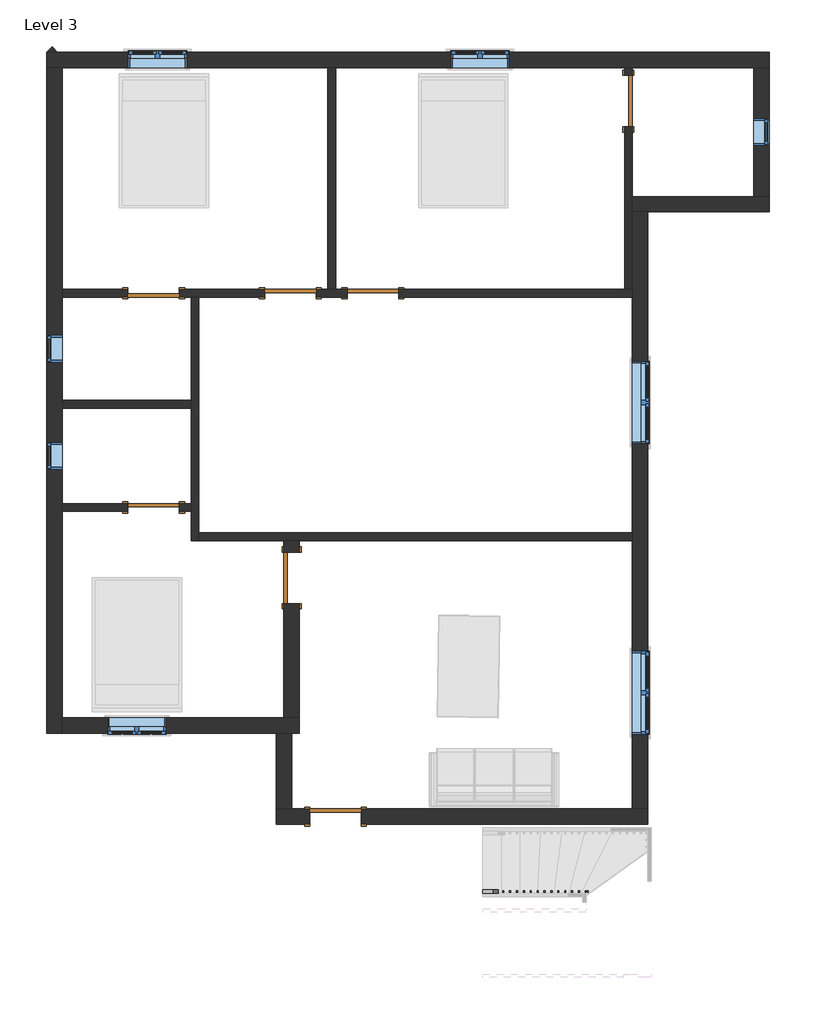
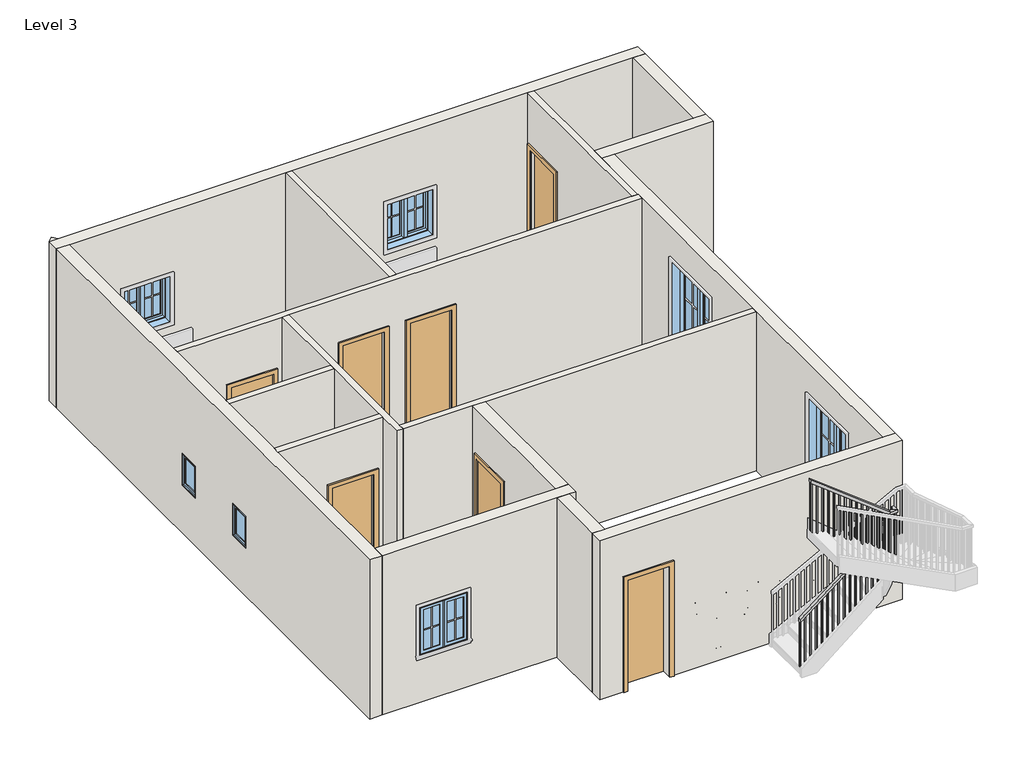
# One storey, part 1 of 2: 17 walls, 8 windows, 7 doors, 1 railing.
"""IFC4 building model written with IfcOpenShell, lengths in millimetres."""

from ifc_helpers import new_model, si_unit, frame, origin, place, context, project, spatial, polyline, outline, extrude, faceted_brep, transform, mapped, element, save
from components import door_f2b275c1, door_d8f5dbb5, door_214872d5, door_78caadf7, door_bb98abfd, window_aa618e30, window_339605e1, window_8377141f

model = new_model("IFC4")

# Units and contexts
model_context = context("Model", 3, world=origin())
ifc_project = project(units=[si_unit("LENGTHUNIT", "METRE", prefix="MILLI")], contexts=[model_context])

# Site, building, storey
site = spatial("IfcSite", under=ifc_project)
building = spatial("IfcBuilding", under=site)
storey = spatial("IfcBuildingStorey", under=building, Name="Level 3", Elevation=3200.4)

# Doors
placement = place(None, origin())
door_shape = door_f2b275c1(model_context)
element("IfcDoor", 1, ObjectType="Single-Flush : 30\" x 80\"", at=placement, inside=storey, context=model_context, shape_type="MappedRepresentation", body=[
    mapped(door_shape, transform((2459.5084916, 7319.9935985, 3200.4), x_axis=(0.0, 1.0, 0.0), y_axis=(-1.0, 0.0, 0.0), z_axis=(0.0, 0.0, 1.0))),
])
element("IfcDoor", 2, ObjectType="Single-Flush : 30\" x 80\"", at=placement, inside=storey, context=model_context, shape_type="MappedRepresentation", body=[
    mapped(door_shape, transform((-4550.8915084, 4481.5435985, 3200.4), x_axis=(1.0, 0.0, 0.0), y_axis=(0.0, 1.0, 0.0), z_axis=(0.0, 0.0, 1.0))),
])
door_2_shape = door_d8f5dbb5(model_context)
element("IfcDoor", 3, ObjectType="Single-Flush : 30\" x 80\"", at=placement, inside=storey, context=model_context, shape_type="MappedRepresentation", body=[
    mapped(door_2_shape, transform((-4550.8915084, 1319.2435985, 3200.4), x_axis=(1.0, 0.0, 0.0), y_axis=(0.0, 1.0, 0.0), z_axis=(0.0, 0.0, 1.0))),
])
door_3_shape = door_214872d5(model_context)
element("IfcDoor", 4, ObjectType="Single-Flush : 30\" x 84\"", at=placement, inside=storey, context=model_context, shape_type="MappedRepresentation", body=[
    mapped(door_3_shape, transform((-2531.5915084, 4481.5435985, 3200.4), x_axis=(1.0, 0.0, 0.0), y_axis=(0.0, 1.0, 0.0), z_axis=(0.0, 0.0, 1.0))),
])
door_4_shape = door_78caadf7(model_context)
element("IfcDoor", 5, ObjectType="Single-Flush : 30\" x 84\"", at=placement, inside=storey, context=model_context, shape_type="MappedRepresentation", body=[
    mapped(door_4_shape, transform((-1312.3915084, 4481.5435985, 3200.4), x_axis=(-1.0, 0.0, 0.0), y_axis=(0.0, -1.0, 0.0), z_axis=(0.0, 0.0, 1.0))),
])
door_5_shape = door_bb98abfd(model_context)
element("IfcDoor", 6, ObjectType="Single-Flush : 30\" x 84\"", at=placement, inside=storey, context=model_context, shape_type="MappedRepresentation", body=[
    mapped(door_5_shape, transform((-2512.5415084, 277.8435985, 3200.4), x_axis=(0.0, 1.0, 0.0), y_axis=(-1.0, 0.0, 0.0), z_axis=(0.0, 0.0, 1.0))),
])
element("IfcDoor", 7, ObjectType="Single-Flush : 30\" x 84\"", at=placement, inside=storey, context=model_context, shape_type="MappedRepresentation", body=[
    mapped(door_5_shape, transform((-1864.8415084, -3246.4064015, 3200.4), x_axis=(1.0, 0.0, 0.0), y_axis=(0.0, 1.0, 0.0), z_axis=(0.0, 0.0, 1.0))),
])

# Railing
element("IfcRailing", 8, ObjectType="Handrail - Rectangular", at=placement, inside=storey, context=model_context, shape_type="SolidModel", body=[
    faceted_brep([(306.9570026, -4325.9064015, 4284.1333333), (306.9570026, -4325.9064015, 4219.8000346), (306.9570026, -4376.7064015, 4219.8000346), (306.9570026, -4376.7064015, 4284.1333333), (1758.4886944, -4325.9064015, 5412.0191036), (1809.2886944, -4325.9064015, 5387.1590024), (1809.2886944, -4376.7064015, 5387.1590024), (1758.4886944, -4376.7064015, 5412.0191036), (1758.4886944, -4325.9064015, 5615.0281882), (1809.2886944, -4325.9064015, 5564.2281882), (1809.2886944, -4376.7064015, 5564.2281882), (1758.4886944, -4376.7064015, 5615.0281882), (1885.4886944, -4325.9064015, 5615.0281882), (1885.4886944, -4325.9064015, 5564.2281882), (1834.6886944, -4376.7064015, 5564.2281882), (1834.6886944, -4376.7064015, 5615.0281882), (1885.4886944, -4452.9064015, 5615.0281882), (1885.4886944, -4482.0277354, 5564.2281882), (1834.6886944, -4482.0277354, 5564.2281882), (1834.6886944, -4452.9064015, 5615.0281882), (1885.4886944, -4579.9064015, 5831.9051451), (1885.4886944, -4630.7064015, 5818.1256424), (1834.6886944, -4630.7064015, 5818.1256424), (1834.6886944, -4579.9064015, 5831.9051451), (1885.4886944, -4579.9064015, 6034.9142297), (1885.4886944, -4630.7064015, 5984.1142297), (1834.6886944, -4630.7064015, 5984.1142297), (1834.6886944, -4579.9064015, 6034.9142297), (1885.4886944, -4706.9064015, 6034.9142297), (1885.4886944, -4706.9064015, 5984.1142297), (1834.6886944, -4656.1064015, 5984.1142297), (1834.6886944, -4656.1064015, 6034.9142297), (1758.4886944, -4706.9064015, 6034.9142297), (1741.0720265, -4706.9064015, 5984.1142297), (1741.0720265, -4656.1064015, 5984.1142297), (1758.4886944, -4656.1064015, 6034.9142297), (306.9570026, -4706.9064015, 7162.8), (306.9570026, -4656.1064015, 7162.8), (306.9570026, -4656.1064015, 7098.4667013), (306.9570026, -4706.9064015, 7098.4667013)], [[[0, 1, 2, 3]], [[1, 0, 4, 5]], [[2, 1, 5, 6]], [[3, 2, 6, 7]], [[0, 3, 7, 4]], [[5, 4, 8, 9]], [[6, 5, 9, 10]], [[7, 6, 10, 11]], [[4, 7, 11, 8]], [[9, 8, 12, 13]], [[10, 9, 13, 14]], [[11, 10, 14, 15]], [[8, 11, 15, 12]], [[13, 12, 16, 17]], [[14, 13, 17, 18]], [[15, 14, 18, 19]], [[12, 15, 19, 16]], [[17, 16, 20, 21]], [[18, 17, 21, 22]], [[19, 18, 22, 23]], [[16, 19, 23, 20]], [[21, 20, 24, 25]], [[22, 21, 25, 26]], [[23, 22, 26, 27]], [[20, 23, 27, 24]], [[25, 24, 28, 29]], [[26, 25, 29, 30]], [[27, 26, 30, 31]], [[24, 27, 31, 28]], [[29, 28, 32, 33]], [[30, 29, 33, 34]], [[31, 30, 34, 35]], [[28, 31, 35, 32]], [[36, 37, 38, 39]], [[33, 32, 36, 39]], [[34, 33, 39, 38]], [[35, 34, 38, 37]], [[32, 35, 37, 36]]]),
    extrude(outline(polyline([(7068.4292361, 345.6136944), (7083.2316852, 326.5636944), (6079.0666667, 326.5636944), (6079.0666667, 345.6136944), (7068.4292361, 345.6136944)])), frame((0.0, -4691.0314015, 0.0), z_axis=(0.0, 1.0, 0.0), x_axis=(0.0, 0.0, 1.0)), (0.0, 0.0, 1.0), 19.05),
    extrude(outline(polyline([(6989.4828411, 447.2136944), (7004.2852902, 428.1636944), (6079.0666667, 428.1636944), (6079.0666667, 447.2136944), (6989.4828411, 447.2136944)])), frame((0.0, -4691.0314015, 0.0), z_axis=(0.0, 1.0, 0.0), x_axis=(0.0, 0.0, 1.0)), (0.0, 0.0, 1.0), 19.05),
    extrude(outline(polyline([(6910.5364462, 548.8136944), (6925.3388952, 529.7636944), (6079.0666667, 529.7636944), (6079.0666667, 548.8136944), (6910.5364462, 548.8136944)])), frame((0.0, -4691.0314015, 0.0), z_axis=(0.0, 1.0, 0.0), x_axis=(0.0, 0.0, 1.0)), (0.0, 0.0, 1.0), 19.05),
    extrude(outline(polyline([(6831.5900512, 650.4136944), (6846.3925003, 631.3636944), (5909.7333333, 631.3636944), (5909.7333333, 650.4136944), (6831.5900512, 650.4136944)])), frame((0.0, -4691.0314015, 0.0), z_axis=(0.0, 1.0, 0.0), x_axis=(0.0, 0.0, 1.0)), (0.0, 0.0, 1.0), 19.05),
    extrude(outline(polyline([(6752.6436562, 752.0136944), (6767.4461053, 732.9636944), (5909.7333333, 732.9636944), (5909.7333333, 752.0136944), (6752.6436562, 752.0136944)])), frame((0.0, -4691.0314015, 0.0), z_axis=(0.0, 1.0, 0.0), x_axis=(0.0, 0.0, 1.0)), (0.0, 0.0, 1.0), 19.05),
    extrude(outline(polyline([(6673.6972613, 853.6136944), (6688.4997103, 834.5636944), (5909.7333333, 834.5636944), (5909.7333333, 853.6136944), (6673.6972613, 853.6136944)])), frame((0.0, -4691.0314015, 0.0), z_axis=(0.0, 1.0, 0.0), x_axis=(0.0, 0.0, 1.0)), (0.0, 0.0, 1.0), 19.05),
    extrude(outline(polyline([(6594.7508663, 955.2136944), (6609.5533154, 936.1636944), (5740.4, 936.1636944), (5740.4, 955.2136944), (6594.7508663, 955.2136944)])), frame((0.0, -4691.0314015, 0.0), z_axis=(0.0, 1.0, 0.0), x_axis=(0.0, 0.0, 1.0)), (0.0, 0.0, 1.0), 19.05),
    extrude(outline(polyline([(6515.8044713, 1056.8136944), (6530.6069204, 1037.7636944), (5740.4, 1037.7636944), (5740.4, 1056.8136944), (6515.8044713, 1056.8136944)])), frame((0.0, -4691.0314015, 0.0), z_axis=(0.0, 1.0, 0.0), x_axis=(0.0, 0.0, 1.0)), (0.0, 0.0, 1.0), 19.05),
    extrude(outline(polyline([(6436.8580764, 1158.4136944), (6451.6605254, 1139.3636944), (5571.0666667, 1139.3636944), (5571.0666667, 1158.4136944), (6436.8580764, 1158.4136944)])), frame((0.0, -4691.0314015, 0.0), z_axis=(0.0, 1.0, 0.0), x_axis=(0.0, 0.0, 1.0)), (0.0, 0.0, 1.0), 19.05),
    extrude(outline(polyline([(6357.9116814, 1260.0136944), (6372.7141304, 1240.9636944), (5571.0666667, 1240.9636944), (5571.0666667, 1260.0136944), (6357.9116814, 1260.0136944)])), frame((0.0, -4691.0314015, 0.0), z_axis=(0.0, 1.0, 0.0), x_axis=(0.0, 0.0, 1.0)), (0.0, 0.0, 1.0), 19.05),
    extrude(outline(polyline([(6278.9652864, 1361.6136944), (6293.7677355, 1342.5636944), (5571.0666667, 1342.5636944), (5571.0666667, 1361.6136944), (6278.9652864, 1361.6136944)])), frame((0.0, -4691.0314015, 0.0), z_axis=(0.0, 1.0, 0.0), x_axis=(0.0, 0.0, 1.0)), (0.0, 0.0, 1.0), 19.05),
    extrude(outline(polyline([(6200.0188914, 1463.2136944), (6214.8213405, 1444.1636944), (5401.7333333, 1444.1636944), (5401.7333333, 1463.2136944), (6200.0188914, 1463.2136944)])), frame((0.0, -4691.0314015, 0.0), z_axis=(0.0, 1.0, 0.0), x_axis=(0.0, 0.0, 1.0)), (0.0, 0.0, 1.0), 19.05),
    extrude(outline(polyline([(6121.0724965, 1564.8136944), (6135.8749455, 1545.7636944), (5401.7333333, 1545.7636944), (5401.7333333, 1564.8136944), (6121.0724965, 1564.8136944)])), frame((0.0, -4691.0314015, 0.0), z_axis=(0.0, 1.0, 0.0), x_axis=(0.0, 0.0, 1.0)), (0.0, 0.0, 1.0), 19.05),
    extrude(outline(polyline([(6042.1261015, 1666.4136944), (6056.9285506, 1647.3636944), (5232.4, 1647.3636944), (5232.4, 1666.4136944), (6042.1261015, 1666.4136944)])), frame((0.0, -4691.0314015, 0.0), z_axis=(0.0, 1.0, 0.0), x_axis=(0.0, 0.0, 1.0)), (0.0, 0.0, 1.0), 19.05),
    extrude(outline(polyline([(5963.1797065, 1768.0136944), (5977.9821556, 1748.9636944), (5232.4, 1748.9636944), (5232.4, 1768.0136944), (5963.1797065, 1768.0136944)])), frame((0.0, -4691.0314015, 0.0), z_axis=(0.0, 1.0, 0.0), x_axis=(0.0, 0.0, 1.0)), (0.0, 0.0, 1.0), 19.05),
    extrude(outline(polyline([(1850.5636944, -4646.5814015), (1869.6136944, -4646.5814015), (1869.6136944, -4665.6314015), (1850.5636944, -4665.6314015), (1850.5636944, -4646.5814015)])), frame((0.0, 0.0, 4893.7333333), z_axis=(0.0, 0.0, 1.0), x_axis=(1.0, 0.0, 0.0)), (0.0, 0.0, 1.0), 1090.3808964),
    extrude(outline(polyline([(-4564.0314015, 5704.26524), (-4544.9814015, 5671.7336964), (-4544.9814015, 4724.4), (-4564.0314015, 4724.4), (-4564.0314015, 5704.26524)])), frame((1850.5636944, 0.0, 0.0), z_axis=(1.0, 0.0, 0.0), x_axis=(0.0, 1.0, 0.0)), (0.0, 0.0, 1.0), 19.05),
    extrude(outline(polyline([(-4462.4314015, 5530.7636744), (-4443.3814015, 5498.2321309), (-4443.3814015, 4555.0666667), (-4462.4314015, 4555.0666667), (-4462.4314015, 5530.7636744)])), frame((1850.5636944, 0.0, 0.0), z_axis=(1.0, 0.0, 0.0), x_axis=(0.0, 1.0, 0.0)), (0.0, 0.0, 1.0), 19.05),
    extrude(outline(polyline([(1821.4320026, -4360.8314015), (1821.4320026, -4341.7814015), (1840.4820026, -4341.7814015), (1840.4820026, -4360.8314015), (1821.4320026, -4360.8314015)])), frame((0.0, 0.0, 4385.7333333), z_axis=(0.0, 0.0, 1.0), x_axis=(1.0, 0.0, 0.0)), (0.0, 0.0, 1.0), 1178.4948549),
    extrude(outline(polyline([(5332.4507888, 1738.8820026), (5317.6483397, 1719.8320026), (4216.4, 1719.8320026), (4216.4, 1738.8820026), (5332.4507888, 1738.8820026)])), frame((0.0, -4360.8314015, 0.0), z_axis=(0.0, 1.0, 0.0), x_axis=(0.0, 0.0, 1.0)), (0.0, 0.0, 1.0), 19.05),
    extrude(outline(polyline([(5253.5043938, 1637.2820026), (5238.7019447, 1618.2320026), (4216.4, 1618.2320026), (4216.4, 1637.2820026), (5253.5043938, 1637.2820026)])), frame((0.0, -4360.8314015, 0.0), z_axis=(0.0, 1.0, 0.0), x_axis=(0.0, 0.0, 1.0)), (0.0, 0.0, 1.0), 19.05),
    extrude(outline(polyline([(5174.5579988, 1535.6820026), (5159.7555498, 1516.6320026), (4047.0666667, 1516.6320026), (4047.0666667, 1535.6820026), (5174.5579988, 1535.6820026)])), frame((0.0, -4360.8314015, 0.0), z_axis=(0.0, 1.0, 0.0), x_axis=(0.0, 0.0, 1.0)), (0.0, 0.0, 1.0), 19.05),
    extrude(outline(polyline([(5095.6116039, 1434.0820026), (5080.8091548, 1415.0320026), (4047.0666667, 1415.0320026), (4047.0666667, 1434.0820026), (5095.6116039, 1434.0820026)])), frame((0.0, -4360.8314015, 0.0), z_axis=(0.0, 1.0, 0.0), x_axis=(0.0, 0.0, 1.0)), (0.0, 0.0, 1.0), 19.05),
    extrude(outline(polyline([(5016.6652089, 1332.4820026), (5001.8627598, 1313.4320026), (3877.7333333, 1313.4320026), (3877.7333333, 1332.4820026), (5016.6652089, 1332.4820026)])), frame((0.0, -4360.8314015, 0.0), z_axis=(0.0, 1.0, 0.0), x_axis=(0.0, 0.0, 1.0)), (0.0, 0.0, 1.0), 19.05),
    extrude(outline(polyline([(4937.7188139, 1230.8820026), (4922.9163649, 1211.8320026), (3877.7333333, 1211.8320026), (3877.7333333, 1230.8820026), (4937.7188139, 1230.8820026)])), frame((0.0, -4360.8314015, 0.0), z_axis=(0.0, 1.0, 0.0), x_axis=(0.0, 0.0, 1.0)), (0.0, 0.0, 1.0), 19.05),
    extrude(outline(polyline([(4858.7724189, 1129.2820026), (4843.9699699, 1110.2320026), (3708.4, 1110.2320026), (3708.4, 1129.2820026), (4858.7724189, 1129.2820026)])), frame((0.0, -4360.8314015, 0.0), z_axis=(0.0, 1.0, 0.0), x_axis=(0.0, 0.0, 1.0)), (0.0, 0.0, 1.0), 19.05),
    extrude(outline(polyline([(4779.826024, 1027.6820026), (4765.0235749, 1008.6320026), (3708.4, 1008.6320026), (3708.4, 1027.6820026), (4779.826024, 1027.6820026)])), frame((0.0, -4360.8314015, 0.0), z_axis=(0.0, 1.0, 0.0), x_axis=(0.0, 0.0, 1.0)), (0.0, 0.0, 1.0), 19.05),
    extrude(outline(polyline([(4700.879629, 926.0820026), (4686.0771799, 907.0320026), (3708.4, 907.0320026), (3708.4, 926.0820026), (4700.879629, 926.0820026)])), frame((0.0, -4360.8314015, 0.0), z_axis=(0.0, 1.0, 0.0), x_axis=(0.0, 0.0, 1.0)), (0.0, 0.0, 1.0), 19.05),
    extrude(outline(polyline([(4621.933234, 824.4820026), (4607.130785, 805.4320026), (3539.0666667, 805.4320026), (3539.0666667, 824.4820026), (4621.933234, 824.4820026)])), frame((0.0, -4360.8314015, 0.0), z_axis=(0.0, 1.0, 0.0), x_axis=(0.0, 0.0, 1.0)), (0.0, 0.0, 1.0), 19.05),
    extrude(outline(polyline([(4542.9868391, 722.8820026), (4528.18439, 703.8320026), (3539.0666667, 703.8320026), (3539.0666667, 722.8820026), (4542.9868391, 722.8820026)])), frame((0.0, -4360.8314015, 0.0), z_axis=(0.0, 1.0, 0.0), x_axis=(0.0, 0.0, 1.0)), (0.0, 0.0, 1.0), 19.05),
    extrude(outline(polyline([(4464.0404441, 621.2820026), (4449.237995, 602.2320026), (3539.0666667, 602.2320026), (3539.0666667, 621.2820026), (4464.0404441, 621.2820026)])), frame((0.0, -4360.8314015, 0.0), z_axis=(0.0, 1.0, 0.0), x_axis=(0.0, 0.0, 1.0)), (0.0, 0.0, 1.0), 19.05),
    extrude(outline(polyline([(4385.0940491, 519.6820026), (4370.2916001, 500.6320026), (3369.7333333, 500.6320026), (3369.7333333, 519.6820026), (4385.0940491, 519.6820026)])), frame((0.0, -4360.8314015, 0.0), z_axis=(0.0, 1.0, 0.0), x_axis=(0.0, 0.0, 1.0)), (0.0, 0.0, 1.0), 19.05),
    extrude(outline(polyline([(4306.1476541, 418.0820026), (4291.3452051, 399.0320026), (3369.7333333, 399.0320026), (3369.7333333, 418.0820026), (4306.1476541, 418.0820026)])), frame((0.0, -4360.8314015, 0.0), z_axis=(0.0, 1.0, 0.0), x_axis=(0.0, 0.0, 1.0)), (0.0, 0.0, 1.0), 19.05),
    extrude(outline(polyline([(1850.5636944, -4671.9814015), (1869.6136944, -4671.9814015), (1869.6136944, -4691.0314015), (1850.5636944, -4691.0314015), (1850.5636944, -4671.9814015)])), frame((0.0, 0.0, 5063.0666667), z_axis=(0.0, 0.0, 1.0), x_axis=(1.0, 0.0, 0.0)), (0.0, 0.0, 1.0), 921.0475631),
    extrude(outline(polyline([(1850.5636944, -4360.8314015), (1850.5636944, -4341.7814015), (1869.6136944, -4341.7814015), (1869.6136944, -4360.8314015), (1850.5636944, -4360.8314015)])), frame((0.0, 0.0, 4385.7333333), z_axis=(0.0, 0.0, 1.0), x_axis=(1.0, 0.0, 0.0)), (0.0, 0.0, 1.0), 1178.4948549),
    extrude(outline(polyline([(7083.6642523, 326.0070026), (7098.4667013, 306.9570026), (6079.0666667, 306.9570026), (6079.0666667, 326.0070026), (7083.6642523, 326.0070026)])), frame((0.0, -4691.0314015, 0.0), z_axis=(0.0, 1.0, 0.0), x_axis=(0.0, 0.0, 1.0)), (0.0, 0.0, 1.0), 19.05),
    extrude(outline(polyline([(4234.6024837, 326.0070026), (4219.8000346, 306.9570026), (3369.7333333, 306.9570026), (3369.7333333, 326.0070026), (4234.6024837, 326.0070026)])), frame((0.0, -4360.8314015, 0.0), z_axis=(0.0, 1.0, 0.0), x_axis=(0.0, 0.0, 1.0)), (0.0, 0.0, 1.0), 19.05),
])

# Walls
element("IfcWall", 9, ObjectType="WALL4.5\"", at=placement, inside=storey, context=model_context, shape_type="SweptSolid", body=[
    extrude(outline(polyline([(-1979.1415084, 4538.6935985), (-1979.1415084, 7815.2935985), (-1864.8415084, 7815.2935985), (-1864.8415084, 4538.6935985), (-1979.1415084, 4538.6935985)])), frame((0.0, 0.0, 3200.4), z_axis=(0.0, 0.0, 1.0), x_axis=(1.0, 0.0, 0.0)), (0.0, 0.0, 1.0), 3048.0),
])
element("IfcWall", 10, ObjectType="WALL4.5\"", at=placement, inside=storey, context=model_context, shape_type="Brep", body=[
    faceted_brep([(-2150.5915084, 4424.3935985, 3200.4), (-1693.3915084, 4424.3935985, 3200.4), (-1693.3915084, 4424.3935985, 5334.0), (-931.3915084, 4424.3935985, 5334.0), (-931.3915084, 4424.3935985, 3200.4), (2516.6584916, 4424.3935985, 3200.4), (2516.6584916, 4424.3935985, 6248.4), (-3884.1415084, 4424.3935985, 6248.4), (-3998.4415084, 4424.3935985, 6248.4), (-5903.4415084, 4424.3935985, 6248.4), (-5903.4415084, 4424.3935985, 3200.4), (-4931.8915084, 4424.3935985, 3200.4), (-4931.8915084, 4424.3935985, 5232.4), (-4169.8915084, 4424.3935985, 5232.4), (-4169.8915084, 4424.3935985, 3200.4), (-3998.4415084, 4424.3935985, 3200.4), (-3884.1415084, 4424.3935985, 3200.4), (-2912.5915084, 4424.3935985, 3200.4), (-2912.5915084, 4424.3935985, 5334.0), (-2150.5915084, 4424.3935985, 5334.0), (-1693.3915084, 4538.6935985, 5334.0), (-1693.3915084, 4538.6935985, 3200.4), (-1864.8415084, 4538.6935985, 3200.4), (-1979.1415084, 4538.6935985, 3200.4), (-2150.5915084, 4538.6935985, 3200.4), (-2150.5915084, 4538.6935985, 5334.0), (-2912.5915084, 4538.6935985, 5334.0), (-2912.5915084, 4538.6935985, 3200.4), (-4169.8915084, 4538.6935985, 3200.4), (-4169.8915084, 4538.6935985, 5232.4), (-4931.8915084, 4538.6935985, 5232.4), (-4931.8915084, 4538.6935985, 3200.4), (-5903.4415084, 4538.6935985, 3200.4), (-5903.4415084, 4538.6935985, 6248.4), (-1979.1415084, 4538.6935985, 6248.4), (-1864.8415084, 4538.6935985, 6248.4), (2402.3584916, 4538.6935985, 6248.4), (2516.6584916, 4538.6935985, 6248.4), (2516.6584916, 4538.6935985, 3200.4), (2402.3584916, 4538.6935985, 3200.4), (-931.3915084, 4538.6935985, 3200.4), (-931.3915084, 4538.6935985, 5334.0)], [[[0, 1, 2, 3, 4, 5, 6, 7, 8, 9, 10, 11, 12, 13, 14, 15, 16, 17, 18, 19]], [[20, 21, 22, 23, 24, 25, 26, 27, 28, 29, 30, 31, 32, 33, 34, 35, 36, 37, 38, 39, 40, 41]], [[11, 10, 32, 31]], [[17, 16, 15, 14, 28, 27]], [[40, 39, 38, 5, 4]], [[24, 23, 22, 21, 1, 0]], [[10, 9, 33, 32]], [[6, 5, 38, 37]], [[29, 28, 14, 13]], [[30, 29, 13, 12]], [[31, 30, 12, 11]], [[25, 24, 0, 19]], [[26, 25, 19, 18]], [[27, 26, 18, 17]], [[2, 1, 21, 20]], [[3, 2, 20, 41]], [[4, 3, 41, 40]], [[9, 8, 7, 6, 37, 36, 35, 34, 33]]]),
])
element("IfcWall", 11, ObjectType="WALL4.5\"", at=placement, inside=storey, context=model_context, shape_type="Brep", body=[
    faceted_brep([(2516.6584916, 7700.9935985, 5232.4), (2516.6584916, 7700.9935985, 3200.4), (2516.6584916, 7815.2935985, 3200.4), (2516.6584916, 7815.2935985, 6248.4), (2516.6584916, 5910.2935985, 6248.4), (2516.6584916, 5681.6935985, 6248.4), (2516.6584916, 4538.6935985, 6248.4), (2516.6584916, 4538.6935985, 3200.4), (2516.6584916, 5681.6935985, 3200.4), (2516.6584916, 5910.2935985, 3200.4), (2516.6584916, 6938.9935985, 3200.4), (2516.6584916, 6938.9935985, 5232.4), (2402.3584916, 7815.2935985, 3200.4), (2402.3584916, 7700.9935985, 3200.4), (2402.3584916, 7700.9935985, 5232.4), (2402.3584916, 6938.9935985, 5232.4), (2402.3584916, 6938.9935985, 3200.4), (2402.3584916, 4538.6935985, 3200.4), (2402.3584916, 4538.6935985, 6248.4), (2402.3584916, 7815.2935985, 6248.4)], [[[0, 1, 2, 3, 4, 5, 6, 7, 8, 9, 10, 11]], [[12, 13, 14, 15, 16, 17, 18, 19]], [[2, 1, 13, 12]], [[10, 9, 8, 7, 17, 16]], [[7, 6, 18, 17]], [[3, 2, 12, 19]], [[14, 13, 1, 0]], [[15, 14, 0, 11]], [[16, 15, 11, 10]], [[6, 5, 4, 3, 19, 18]]]),
])
element("IfcWall", 12, ObjectType="WALL4.5\"", at=placement, inside=storey, context=model_context, shape_type="Brep", body=[
    faceted_brep([(-3998.4415084, 4424.3935985, 3200.4), (-3998.4415084, 2900.3935985, 3200.4), (-3998.4415084, 2786.0935985, 3200.4), (-3998.4415084, 1376.3935985, 3200.4), (-3998.4415084, 1262.0935985, 3200.4), (-3998.4415084, 830.2935985, 3200.4), (-3998.4415084, 830.2935985, 6248.4), (-3998.4415084, 1262.0935985, 6248.4), (-3998.4415084, 1376.3935985, 6248.4), (-3998.4415084, 2786.0935985, 6248.4), (-3998.4415084, 2900.3935985, 6248.4), (-3998.4415084, 4424.3935985, 6248.4), (-3884.1415084, 4424.3935985, 3200.4), (-3884.1415084, 4424.3935985, 6248.4), (-3884.1415084, 944.5935985, 6248.4), (-3884.1415084, 830.2935985, 6248.4), (-3884.1415084, 830.2935985, 3200.4), (-3884.1415084, 944.5935985, 3200.4)], [[[0, 1, 2, 3, 4, 5, 6, 7, 8, 9, 10, 11]], [[12, 13, 14, 15, 16, 17]], [[5, 4, 3, 2, 1, 0, 12, 17, 16]], [[0, 11, 13, 12]], [[6, 5, 16, 15]], [[11, 10, 9, 8, 7, 6, 15, 14, 13]]]),
])
element("IfcWall", 13, ObjectType="WALL4.5\"", at=placement, inside=storey, context=model_context, shape_type="Brep", body=[
    faceted_brep([(-3884.1415084, 830.2935985, 3200.4), (-2626.8415084, 830.2935985, 3200.4), (-2398.2415084, 830.2935985, 3200.4), (2516.6584916, 830.2935985, 3200.4), (2516.6584916, 830.2935985, 6248.4), (-2398.2415084, 830.2935985, 6248.4), (-2626.8415084, 830.2935985, 6248.4), (-3884.1415084, 830.2935985, 6248.4), (-3884.1415084, 944.5935985, 3200.4), (-3884.1415084, 944.5935985, 6248.4), (2516.6584916, 944.5935985, 6248.4), (2516.6584916, 944.5935985, 3200.4)], [[[0, 1, 2, 3, 4, 5, 6, 7]], [[8, 9, 10, 11]], [[3, 2, 1, 0, 8, 11]], [[0, 7, 9, 8]], [[4, 3, 11, 10]], [[7, 6, 5, 4, 10, 9]]]),
])
element("IfcWall", 14, ObjectType="WALL4.5\"", at=placement, inside=storey, context=model_context, shape_type="SweptSolid", body=[
    extrude(outline(polyline([(-3998.4415084, 2786.0935985), (-5903.4415084, 2786.0935985), (-5903.4415084, 2900.3935985), (-3998.4415084, 2900.3935985), (-3998.4415084, 2786.0935985)])), frame((0.0, 0.0, 3200.4), z_axis=(0.0, 0.0, 1.0), x_axis=(1.0, 0.0, 0.0)), (0.0, 0.0, 1.0), 3048.0),
])
element("IfcWall", 15, ObjectType="WALL4.5\"", at=placement, inside=storey, context=model_context, shape_type="SweptSolid", body=[
    extrude(outline(polyline([(5232.4, -4169.8915084), (3200.4, -4169.8915084), (3200.4, -3998.4415084), (6248.4, -3998.4415084), (6248.4, -5903.4415084), (3200.4, -5903.4415084), (3200.4, -4931.8915084), (5232.4, -4931.8915084), (5232.4, -4169.8915084)])), frame((0.0, 1262.0935985, 0.0), z_axis=(0.0, 1.0, 0.0), x_axis=(0.0, 0.0, 1.0)), (0.0, 0.0, 1.0), 114.3),
])
element("IfcWall", 16, ObjectType="WALL4.5\"", at=placement, inside=storey, context=model_context, shape_type="SweptSolid", body=[
    extrude(outline(polyline([(-6051.2188015, 8124.7159036), (-5970.3964964, 8043.8935985), (-6132.0411066, 8043.8935985), (-6051.2188015, 8124.7159036)])), frame((0.0, 0.0, 3200.4), z_axis=(0.0, 0.0, 1.0), x_axis=(1.0, 0.0, 0.0)), (0.0, 0.0, 1.0), 3048.0),
])
element("IfcWall", 17, ObjectType="WALL9\"", at=placement, inside=storey, context=model_context, shape_type="Brep", body=[
    faceted_brep([(-6132.0415084, 7815.2935985, 3200.4), (-5903.4415084, 7815.2935985, 3200.4), (-1979.1415084, 7815.2935985, 3200.4), (-1864.8415084, 7815.2935985, 3200.4), (2402.3584916, 7815.2935985, 3200.4), (2516.6584916, 7815.2935985, 3200.4), (4307.3584916, 7815.2935985, 3200.4), (4535.9584916, 7815.2935985, 3200.4), (4535.9584916, 7815.2935985, 6248.4), (4307.3584916, 7815.2935985, 6248.4), (2516.6584916, 7815.2935985, 6248.4), (2402.3584916, 7815.2935985, 6248.4), (-1864.8415084, 7815.2935985, 6248.4), (-1979.1415084, 7815.2935985, 6248.4), (-5903.4415084, 7815.2935985, 6248.4), (-6132.0415084, 7815.2935985, 6248.4), (-4061.9415084, 7815.2935985, 5029.2), (-4061.9415084, 7815.2935985, 4114.8), (-4925.5415084, 7815.2935985, 4114.8), (-4925.5415084, 7815.2935985, 5029.2), (700.5584916, 7815.2935985, 5029.2), (700.5584916, 7815.2935985, 4114.8), (-163.0415084, 7815.2935985, 4114.8), (-163.0415084, 7815.2935985, 5029.2), (-6132.0415084, 8043.8935985, 3200.4), (-6132.0415084, 8043.8935985, 6248.4), (-5970.3964964, 8043.8935985, 6248.4), (4535.9584916, 8043.8935985, 6248.4), (4535.9584916, 8043.8935985, 3200.4), (-5970.3964964, 8043.8935985, 3200.4), (-4061.9415084, 8043.8935985, 5029.2), (-4925.5415084, 8043.8935985, 5029.2), (-4925.5415084, 8043.8935985, 4114.8), (-4061.9415084, 8043.8935985, 4114.8), (700.5584916, 8043.8935985, 5029.2), (-163.0415084, 8043.8935985, 5029.2), (-163.0415084, 8043.8935985, 4114.8), (700.5584916, 8043.8935985, 4114.8)], [[[0, 1, 2, 3, 4, 5, 6, 7, 8, 9, 10, 11, 12, 13, 14, 15], [16, 17, 18, 19], [20, 21, 22, 23]], [[24, 25, 26, 27, 28, 29], [30, 31, 32, 33], [34, 35, 36, 37]], [[7, 6, 5, 4, 3, 2, 1, 0, 24, 29, 28]], [[0, 15, 25, 24]], [[8, 7, 28, 27]], [[17, 16, 30, 33]], [[18, 17, 33, 32]], [[19, 18, 32, 31]], [[16, 19, 31, 30]], [[21, 20, 34, 37]], [[22, 21, 37, 36]], [[23, 22, 36, 35]], [[20, 23, 35, 34]], [[15, 14, 13, 12, 11, 10, 9, 8, 27, 26, 25]]]),
])
element("IfcWall", 18, ObjectType="WALL9\"", at=placement, inside=storey, context=model_context, shape_type="Brep", body=[
    faceted_brep([(-6132.0415084, 7815.2935985, 3200.4), (-6132.0415084, -2014.5064015, 3200.4), (-6132.0415084, -2014.5064015, 6248.4), (-6132.0415084, 7815.2935985, 6248.4), (-6132.0415084, 3865.5935985, 4724.4), (-6132.0415084, 3459.1935985, 4724.4), (-6132.0415084, 3459.1935985, 4114.8), (-6132.0415084, 3865.5935985, 4114.8), (-6132.0415084, 2284.4435985, 4724.4), (-6132.0415084, 1878.0435985, 4724.4), (-6132.0415084, 1878.0435985, 4114.8), (-6132.0415084, 2284.4435985, 4114.8), (-5903.4415084, 7815.2935985, 3200.4), (-5903.4415084, 7815.2935985, 6248.4), (-5903.4415084, 4538.6935985, 6248.4), (-5903.4415084, 4424.3935985, 6248.4), (-5903.4415084, 2900.3935985, 6248.4), (-5903.4415084, 2786.0935985, 6248.4), (-5903.4415084, 1376.3935985, 6248.4), (-5903.4415084, 1262.0935985, 6248.4), (-5903.4415084, -1785.9064015, 6248.4), (-5903.4415084, -2014.5064015, 6248.4), (-5903.4415084, -2014.5064015, 3200.4), (-5903.4415084, -1785.9064015, 3200.4), (-5903.4415084, 1262.0935985, 3200.4), (-5903.4415084, 1376.3935985, 3200.4), (-5903.4415084, 2786.0935985, 3200.4), (-5903.4415084, 2900.3935985, 3200.4), (-5903.4415084, 4424.3935985, 3200.4), (-5903.4415084, 4538.6935985, 3200.4), (-5903.4415084, 3865.5935985, 4724.4), (-5903.4415084, 3865.5935985, 4114.8), (-5903.4415084, 3459.1935985, 4114.8), (-5903.4415084, 3459.1935985, 4724.4), (-5903.4415084, 2284.4435985, 4724.4), (-5903.4415084, 2284.4435985, 4114.8), (-5903.4415084, 1878.0435985, 4114.8), (-5903.4415084, 1878.0435985, 4724.4)], [[[0, 1, 2, 3], [4, 5, 6, 7], [8, 9, 10, 11]], [[12, 13, 14, 15, 16, 17, 18, 19, 20, 21, 22, 23, 24, 25, 26, 27, 28, 29], [30, 31, 32, 33], [34, 35, 36, 37]], [[1, 0, 12, 29, 28, 27, 26, 25, 24, 23, 22]], [[0, 3, 13, 12]], [[2, 1, 22, 21]], [[31, 30, 4, 7]], [[32, 31, 7, 6]], [[33, 32, 6, 5]], [[30, 33, 5, 4]], [[35, 34, 8, 11]], [[36, 35, 11, 10]], [[37, 36, 10, 9]], [[34, 37, 9, 8]], [[3, 2, 21, 20, 19, 18, 17, 16, 15, 14, 13]]]),
])
element("IfcWall", 19, ObjectType="WALL9\"", at=placement, inside=storey, context=model_context, shape_type="Brep", body=[
    faceted_brep([(-5903.4415084, -2014.5064015, 3200.4), (-2741.1415084, -2014.5064015, 3200.4), (-2512.5415084, -2014.5064015, 3200.4), (-2398.2415084, -2014.5064015, 3200.4), (-2398.2415084, -2014.5064015, 6248.4), (-2512.5415084, -2014.5064015, 6248.4), (-2741.1415084, -2014.5064015, 6248.4), (-5903.4415084, -2014.5064015, 6248.4), (-5230.3415084, -2014.5064015, 5029.2), (-4366.7415084, -2014.5064015, 5029.2), (-4366.7415084, -2014.5064015, 4114.8), (-5230.3415084, -2014.5064015, 4114.8), (-5903.4415084, -1785.9064015, 3200.4), (-5903.4415084, -1785.9064015, 6248.4), (-2626.8415084, -1785.9064015, 6248.4), (-2398.2415084, -1785.9064015, 6248.4), (-2398.2415084, -1785.9064015, 3200.4), (-2626.8415084, -1785.9064015, 3200.4), (-5230.3415084, -1785.9064015, 5029.2), (-5230.3415084, -1785.9064015, 4114.8), (-4366.7415084, -1785.9064015, 4114.8), (-4366.7415084, -1785.9064015, 5029.2)], [[[0, 1, 2, 3, 4, 5, 6, 7], [8, 9, 10, 11]], [[12, 13, 14, 15, 16, 17], [18, 19, 20, 21]], [[3, 2, 1, 0, 12, 17, 16]], [[0, 7, 13, 12]], [[4, 3, 16, 15]], [[19, 18, 8, 11]], [[20, 19, 11, 10]], [[21, 20, 10, 9]], [[18, 21, 9, 8]], [[7, 6, 5, 4, 15, 14, 13]]]),
])
element("IfcWall", 20, ObjectType="WALL9\"", at=placement, inside=storey, context=model_context, shape_type="SweptSolid", body=[
    extrude(outline(polyline([(830.2935985, 3200.4), (658.8435985, 3200.4), (658.8435985, 5334.0), (-103.1564015, 5334.0), (-103.1564015, 3200.4), (-1785.9064015, 3200.4), (-1785.9064015, 6248.4), (830.2935985, 6248.4), (830.2935985, 3200.4)])), frame((-2626.8415084, 0.0, 0.0), z_axis=(1.0, 0.0, 0.0), x_axis=(0.0, 1.0, 0.0)), (0.0, 0.0, 1.0), 228.6),
])
element("IfcWall", 21, ObjectType="WALL9\"", at=placement, inside=storey, context=model_context, shape_type="Brep", body=[
    faceted_brep([(2745.2584916, -3132.1064015, 3200.4), (2516.6584916, -3132.1064015, 3200.4), (-1483.8415084, -3132.1064015, 3200.4), (-1483.8415084, -3132.1064015, 5334.0), (-2245.8415084, -3132.1064015, 5334.0), (-2245.8415084, -3132.1064015, 3200.4), (-2512.5415084, -3132.1064015, 3200.4), (-2741.1415084, -3132.1064015, 3200.4), (-2741.1415084, -3132.1064015, 6248.4), (-2512.5415084, -3132.1064015, 6248.4), (2516.6584916, -3132.1064015, 6248.4), (2745.2584916, -3132.1064015, 6248.4), (-1483.8415084, -3360.7064015, 5334.0), (-1483.8415084, -3360.7064015, 3200.4), (2745.2584916, -3360.7064015, 3200.4), (2745.2584916, -3360.7064015, 6248.4), (-2741.1415084, -3360.7064015, 6248.4), (-2741.1415084, -3360.7064015, 3200.4), (-2245.8415084, -3360.7064015, 3200.4), (-2245.8415084, -3360.7064015, 5334.0)], [[[0, 1, 2, 3, 4, 5, 6, 7, 8, 9, 10, 11]], [[12, 13, 14, 15, 16, 17, 18, 19]], [[18, 17, 7, 6, 5]], [[14, 13, 2, 1, 0]], [[8, 7, 17, 16]], [[0, 11, 15, 14]], [[3, 2, 13, 12]], [[4, 3, 12, 19]], [[5, 4, 19, 18]], [[11, 10, 9, 8, 16, 15]]]),
])
element("IfcWall", 22, ObjectType="WALL9\"", at=placement, inside=storey, context=model_context, shape_type="SweptSolid", body=[
    extrude(outline(polyline([(-2512.5415084, -2014.5064015), (-2512.5415084, -3132.1064015), (-2741.1415084, -3132.1064015), (-2741.1415084, -2014.5064015), (-2512.5415084, -2014.5064015)])), frame((0.0, 0.0, 3200.4), z_axis=(0.0, 0.0, 1.0), x_axis=(1.0, 0.0, 0.0)), (0.0, 0.0, 1.0), 3048.0),
])
element("IfcWall", 23, ObjectType="WALL9\"", at=placement, inside=storey, context=model_context, shape_type="Brep", body=[
    faceted_brep([(4535.9584916, 5910.2935985, 3200.4), (4307.3584916, 5910.2935985, 3200.4), (2516.6584916, 5910.2935985, 3200.4), (2516.6584916, 5910.2935985, 6248.4), (4307.3584916, 5910.2935985, 6248.4), (4535.9584916, 5910.2935985, 6248.4), (4535.9584916, 5681.6935985, 3200.4), (4535.9584916, 5681.6935985, 6248.4), (2745.2584916, 5681.6935985, 6248.4), (2516.6584916, 5681.6935985, 6248.4), (2516.6584916, 5681.6935985, 3200.4), (2745.2584916, 5681.6935985, 3200.4)], [[[0, 1, 2, 3, 4, 5]], [[6, 7, 8, 9, 10, 11]], [[2, 1, 0, 6, 11, 10]], [[3, 2, 10, 9]], [[0, 5, 7, 6]], [[5, 4, 3, 9, 8, 7]]]),
])
element("IfcWall", 24, ObjectType="WALL9\"", at=placement, inside=storey, context=model_context, shape_type="Brep", body=[
    faceted_brep([(2516.6584916, 5681.6935985, 3200.4), (2516.6584916, 944.5935985, 3200.4), (2516.6584916, 830.2935985, 3200.4), (2516.6584916, -3132.1064015, 3200.4), (2516.6584916, -3132.1064015, 6248.4), (2516.6584916, 830.2935985, 6248.4), (2516.6584916, 944.5935985, 6248.4), (2516.6584916, 5681.6935985, 6248.4), (2516.6584916, -2027.2064015, 5638.8), (2516.6584916, -2027.2064015, 4114.8), (2516.6584916, -808.0064015, 4114.8), (2516.6584916, -808.0064015, 5638.8), (2516.6584916, 2259.0435985, 5638.8), (2516.6584916, 2259.0435985, 4114.8), (2516.6584916, 3478.2435985, 4114.8), (2516.6584916, 3478.2435985, 5638.8), (2745.2584916, 5681.6935985, 3200.4), (2745.2584916, 5681.6935985, 6248.4), (2745.2584916, -3132.1064015, 6248.4), (2745.2584916, -3132.1064015, 3200.4), (2745.2584916, -2027.2064015, 5638.8), (2745.2584916, -808.0064015, 5638.8), (2745.2584916, -808.0064015, 4114.8), (2745.2584916, -2027.2064015, 4114.8), (2745.2584916, 2259.0435985, 5638.8), (2745.2584916, 3478.2435985, 5638.8), (2745.2584916, 3478.2435985, 4114.8), (2745.2584916, 2259.0435985, 4114.8)], [[[0, 1, 2, 3, 4, 5, 6, 7], [8, 9, 10, 11], [12, 13, 14, 15]], [[16, 17, 18, 19], [20, 21, 22, 23], [24, 25, 26, 27]], [[3, 2, 1, 0, 16, 19]], [[4, 3, 19, 18]], [[0, 7, 17, 16]], [[9, 8, 20, 23]], [[10, 9, 23, 22]], [[11, 10, 22, 21]], [[8, 11, 21, 20]], [[13, 12, 24, 27]], [[14, 13, 27, 26]], [[15, 14, 26, 25]], [[12, 15, 25, 24]], [[7, 6, 5, 4, 18, 17]]]),
])
element("IfcWall", 25, ObjectType="WALL9\"", at=placement, inside=storey, context=model_context, shape_type="SweptSolid", body=[
    extrude(outline(polyline([(5910.2935985, 3200.4), (5910.2935985, 6248.4), (7815.2935985, 6248.4), (7815.2935985, 3200.4), (5910.2935985, 3200.4)]), holes=[polyline([(6659.5935985, 4724.4), (6659.5935985, 4114.8), (7065.9935985, 4114.8), (7065.9935985, 4724.4), (6659.5935985, 4724.4)])]), frame((4307.3584916, 0.0, 0.0), z_axis=(1.0, 0.0, 0.0), x_axis=(0.0, 1.0, 0.0)), (0.0, 0.0, 1.0), 228.6),
])

# Windows
window_shape = window_aa618e30(model_context)
element("IfcWindow", 26, ObjectType="Fixed : 16\" x 24\"", at=placement, inside=storey, context=model_context, shape_type="MappedRepresentation", body=[
    mapped(window_shape, transform((-6017.7415084, 3700.4935985, 3200.4), x_axis=(0.0, 1.0, 0.0), y_axis=(-1.0, 0.0, 0.0), z_axis=(0.0, 0.0, 1.0))),
])
element("IfcWindow", 27, ObjectType="Fixed : 16\" x 24\"", at=placement, inside=storey, context=model_context, shape_type="MappedRepresentation", body=[
    mapped(window_shape, transform((-6017.7415084, 2119.3435985, 3200.4), x_axis=(0.0, 1.0, 0.0), y_axis=(-1.0, 0.0, 0.0), z_axis=(0.0, 0.0, 1.0))),
])
element("IfcWindow", 28, ObjectType="Fixed : 16\" x 24\"", at=placement, inside=storey, context=model_context, shape_type="MappedRepresentation", body=[
    mapped(window_shape, transform((4421.6584916, 6824.6935985, 3200.4), x_axis=(0.0, -1.0, 0.0), y_axis=(1.0, 0.0, 0.0), z_axis=(0.0, 0.0, 1.0))),
])
window_2_shape = window_339605e1(model_context)
element("IfcWindow", 29, ObjectType="Window-Casement-Double : 34\" x 36\"", at=placement, inside=storey, context=model_context, shape_type="MappedRepresentation", body=[
    mapped(window_2_shape, transform((-4493.7415084, 7929.5935985, 3200.4), x_axis=(1.0, 0.0, 0.0), y_axis=(0.0, 1.0, 0.0), z_axis=(0.0, 0.0, 1.0))),
])
element("IfcWindow", 30, ObjectType="Window-Casement-Double : 34\" x 36\"", at=placement, inside=storey, context=model_context, shape_type="MappedRepresentation", body=[
    mapped(window_2_shape, transform((268.7584916, 7929.5935985, 3200.4), x_axis=(1.0, 0.0, 0.0), y_axis=(0.0, 1.0, 0.0), z_axis=(0.0, 0.0, 1.0))),
])
element("IfcWindow", 31, ObjectType="Window-Casement-Double : 34\" x 36\"", at=placement, inside=storey, context=model_context, shape_type="MappedRepresentation", body=[
    mapped(window_2_shape, transform((-4798.5415084, -1900.2064015, 3200.4), x_axis=(-1.0, 0.0, 0.0), y_axis=(0.0, -1.0, 0.0), z_axis=(0.0, 0.0, 1.0))),
])
window_3_shape = window_8377141f(model_context)
element("IfcWindow", 32, ObjectType="Window-Casement-Double : 48\" x 60\"", at=placement, inside=storey, context=model_context, shape_type="MappedRepresentation", body=[
    mapped(window_3_shape, transform((2630.9584916, -1417.6064015, 3200.4), x_axis=(0.0, -1.0, 0.0), y_axis=(1.0, 0.0, 0.0), z_axis=(0.0, 0.0, 1.0))),
])
element("IfcWindow", 33, ObjectType="Window-Casement-Double : 48\" x 60\"", at=placement, inside=storey, context=model_context, shape_type="MappedRepresentation", body=[
    mapped(window_3_shape, transform((2630.9584916, 2868.6435985, 3200.4), x_axis=(0.0, -1.0, 0.0), y_axis=(1.0, 0.0, 0.0), z_axis=(0.0, 0.0, 1.0))),
])

save(model, "model.ifc")

# Revit data of these elements
# Type "Single-Flush : 30\" x 80\""
#   Type Mark = "5"
#   Construction Type Id = "MDOOR"
#   Assembly Code = "C1020"
#   Analytic Construction = "Metal"
#   Thickness = 0' - 2"
#   Heat Transfer Coefficient (U) = 0.651978 BTU/(h·ft²·°F)
#   Height = 6' - 8"
#   Trim Projection Ext = 0' - 1"
#   Trim Projection Int = 0' - 1"
#   Trim Width = 0' - 3"
#   Width = 2' - 6"
#   Define Thermal Properties by = 1
#   Define Thermal Properties by = 1
#   Door Material = Door - Panel
#   Frame Material = Door - Frame
#   Visual Light Transmittance = 0
#   Solar Heat Gain Coefficient = 0
#   Function = (empty or 0)
#   Wall Closure = (empty or 0)
# Type "Single-Flush : 30\" x 84\""
#   Type Mark = "4"
#   Construction Type Id = "MDOOR"
#   Assembly Code = "C1020"
#   Analytic Construction = "Metal"
#   Thickness = 0' - 2"
#   Heat Transfer Coefficient (U) = 0.651978 BTU/(h·ft²·°F)
#   Height = 7' - 0"
#   Trim Projection Ext = 0' - 1"
#   Trim Projection Int = 0' - 1"
#   Trim Width = 0' - 3"
#   Width = 2' - 6"
#   Define Thermal Properties by = 1
#   Define Thermal Properties by = 1
#   Door Material = Door - Panel
#   Frame Material = Door - Frame
#   Visual Light Transmittance = 0
#   Solar Heat Gain Coefficient = 0
#   Function = (empty or 0)
#   Wall Closure = (empty or 0)
# Type "Handrail - Rectangular"
#   Assembly Code = "C2010400"
#   built-in parameter 1008612 = 0.0416667 (stored number, unit not read)
#   built-in parameter 1008611 = 0.0416667 (stored number, unit not read)
#   built-in parameter 1008609 = 0.333333 (stored number, unit not read)
#   built-in parameter 1008604 = 0.166667 (stored number, unit not read)
#   built-in parameter 1008603 = 0.166667 (stored number, unit not read)
#   Railing Height = 3' - 0"
#   built-in parameter 1008630 = 2
#   built-in parameter 1008610 = 2
#   built-in parameter 1008618 = Baluster - Square : 3/4"
# Type "WALL4.5\""
#   Assembly Code = "B2010"
#   Layers, outside or top first: 0' - 4 1/2" no material (function 1)
# Type "WALL9\""
#   Assembly Code = "B2010"
#   Layers, outside or top first: 0' - 9" no material (function 1)
# Type "Fixed : 16\" x 24\""
#   Type Mark = "4"
#   Construction Type Id = "GSP4R"
#   Assembly Code = "B2020100"
#   Analytic Construction = "1/8 in Pilkington single glazing"
#   Visual Light Transmittance = 0.9
#   Solar Heat Gain Coefficient = 0.78
#   Heat Transfer Coefficient (U) = 0.6496 BTU/(h·ft²·°F)
#   Height = 2' - 0"
#   Default Sill Height = 3' - 0"
#   Width = 1' - 4"
#   Window Inset = 0' - 0 3/4"
#   Define Thermal Properties by = 1
#   Define Thermal Properties by = 1
#   Glass Pane Material = Glass
#   Sash Material = Sash
#   Wall Closure = (empty or 0)
# Type "Window-Casement-Double : 34\" x 36\""
#   Type Mark = "14"
#   Fire Rating = "0.5h"
#   Assembly Code = "B2020100"
#   Analytic Construction = "Double glazing - domestic"
#   Frame Extension [instance default] = 0' - 0 1/4"
#   Window Inset [instance default] = 0' - 0"
#   Wall Thickness [instance default] = 0' - 6"
#   Interior Wall Closure [instance default] = 0' - 2 1/4"
#   Half Width = 1' - 5"
#   Visual Light Transmittance = 0.81
#   Thermal Resistance (R) = 1.8146 (h·ft²·°F)/BTU
#   Solar Heat Gain Coefficient = 0.76
#   Rough Width = 2' - 10 1/2"
#   Rough Height = 3' - 0 1/2"
#   Height = 3' - 0"
#   Heat Transfer Coefficient (U) = 0.5511 BTU/(h·ft²·°F)
#   Exterior Wall Closure [instance default] = 0' - 1 1/4"
#   Extension Jamb [instance default] = 0' - 2 1/4"
#   Default Sill Height = 3' - 0"
#   Width = 2' - 10"
#   Define Thermal Properties by = 0
#   Muntin Visibility = yes
#   Interior Trim Visibility [instance default] = yes
#   Exterior Trim Visibility [instance default] = yes
#   Extension Jamb Visibility [instance default] = yes
#   Interior Trim Material = Wood - Stained
#   Muntin Pattern = Muntin Pattern_2x2 : Muntin Pattern_2x2
#   Interior Trim = Trim-Window-Interior-Flat : Picture Frame
#   Interior Frame Material = Wood - Stained
#   Glass Panel Material = Glass
#   Exterior Trim Material = Clad - White
#   Exterior Trim = Trim-Window-Exterior-Flat : with Sill
#   Exterior Frame Material = Clad - White
#   Wall Closure = (empty or 0)
# Type "Window-Casement-Double : 48\" x 60\""
#   Type Mark = "16"
#   Fire Rating = "0.5h"
#   Assembly Code = "B2020100"
#   Analytic Construction = "Double glazing - domestic"
#   Frame Extension [instance default] = 0' - 0 1/4"
#   Window Inset [instance default] = 0' - 0"
#   Wall Thickness [instance default] = 0' - 6"
#   Interior Wall Closure [instance default] = 0' - 2 1/4"
#   Half Width = 2' - 0"
#   Visual Light Transmittance = 0.81
#   Thermal Resistance (R) = 1.8146 (h·ft²·°F)/BTU
#   Solar Heat Gain Coefficient = 0.76
#   Rough Width = 4' - 0 1/2"
#   Rough Height = 5' - 0 1/2"
#   Height = 5' - 0"
#   Heat Transfer Coefficient (U) = 0.5511 BTU/(h·ft²·°F)
#   Exterior Wall Closure [instance default] = 0' - 1 1/4"
#   Extension Jamb [instance default] = 0' - 2 1/4"
#   Default Sill Height = 3' - 0"
#   Width = 4' - 0"
#   Define Thermal Properties by = 0
#   Muntin Visibility = yes
#   Interior Trim Visibility [instance default] = yes
#   Exterior Trim Visibility [instance default] = yes
#   Extension Jamb Visibility [instance default] = yes
#   Interior Trim Material = Wood - Stained
#   Muntin Pattern = Muntin Pattern_2x2 : Muntin Pattern_2x2
#   Interior Trim = Trim-Window-Interior-Flat : Picture Frame
#   Interior Frame Material = Wood - Stained
#   Glass Panel Material = Glass
#   Exterior Trim Material = Clad - White
#   Exterior Trim = Trim-Window-Exterior-Flat : with Sill
#   Exterior Frame Material = Clad - White
#   Wall Closure = (empty or 0)
# Elements 1, 2, 3 (IfcDoor, "Single-Flush : 30\" x 80\"")
#   Phase Created = New Construction
#   Materials on its faces: "Door - Frame", "Door - Panel"
# Elements 4, 5, 6, 7 (IfcDoor, "Single-Flush : 30\" x 84\"")
#   Phase Created = New Construction
#   Materials on its faces: "Door - Frame", "Door - Panel"
# Element 8 (IfcRailing, "Handrail - Rectangular")
#   Phase Created = New Construction
# Elements 9, 10, 11, 12, 13, 14, 15, 16 (IfcWall, "WALL4.5\"")
#   Top Offset = 0' - 0"
#   Base Offset = 0' - 0"
#   Unconnected Height = 10' - 0"
#   wall height = 10' - 0"
#   Phase Created = New Construction
#   Base Constraint = Level 3
#   Materials on its faces: "Default Wall"
# Elements 17, 18, 19, 21, 22, 23, 24, 25 (IfcWall, "WALL9\"")
#   Top Offset = 0' - 0"
#   Base Offset = 0' - 0"
#   Unconnected Height = 10' - 0"
#   wall height = 10' - 0"
#   Phase Created = New Construction
#   Base Constraint = Level 3
#   Materials on its faces: "Default Wall", "Wood - Stained"
# Element 20 (IfcWall, "WALL9\"")
#   Top Offset = 0' - 0"
#   Base Offset = 0' - 0"
#   Unconnected Height = 10' - 0"
#   wall height = 10' - 0"
#   Phase Created = New Construction
#   Base Constraint = Level 3
#   Materials on its faces: "Default Wall"
# Element 26 (IfcWindow, "Fixed : 16\" x 24\"")
#   Mark = "11"
#   Phase Created = New Construction
#   Materials on its faces: "Sash", "Glass"
# Element 27 (IfcWindow, "Fixed : 16\" x 24\"")
#   Mark = "12"
#   Phase Created = New Construction
#   Materials on its faces: "Sash", "Glass"
# Element 28 (IfcWindow, "Fixed : 16\" x 24\"")
#   Mark = "16"
#   Phase Created = New Construction
#   Materials on its faces: "Sash", "Glass"
# Element 29 (IfcWindow, "Window-Casement-Double : 34\" x 36\"")
#   Mark = "9"
#   Window Inset = 0' - 0"
#   Interior Wall Closure = 0' - 2 1/4"
#   Frame Extension = 0' - 0 1/4"
#   Exterior Wall Closure = 0' - 1 1/4"
#   Interior Trim Visibility = yes
#   Exterior Trim Visibility = yes
#   Phase Created = New Construction
#   Materials on its faces: "Wood - Stained", "Glass", "Clad - White"
# Element 30 (IfcWindow, "Window-Casement-Double : 34\" x 36\"")
#   Mark = "10"
#   Window Inset = 0' - 0"
#   Interior Wall Closure = 0' - 2 1/4"
#   Frame Extension = 0' - 0 1/4"
#   Exterior Wall Closure = 0' - 1 1/4"
#   Interior Trim Visibility = yes
#   Exterior Trim Visibility = yes
#   Phase Created = New Construction
#   Materials on its faces: "Wood - Stained", "Glass", "Clad - White"
# Element 31 (IfcWindow, "Window-Casement-Double : 34\" x 36\"")
#   Mark = "13"
#   Window Inset = 0' - 0"
#   Interior Wall Closure = 0' - 2 1/4"
#   Frame Extension = 0' - 0 1/4"
#   Exterior Wall Closure = 0' - 1 1/4"
#   Interior Trim Visibility = yes
#   Exterior Trim Visibility = yes
#   Phase Created = New Construction
#   Materials on its faces: "Wood - Stained", "Glass", "Clad - White"
# Element 32 (IfcWindow, "Window-Casement-Double : 48\" x 60\"")
#   Mark = "14"
#   Window Inset = 0' - 0"
#   Interior Wall Closure = 0' - 2 1/4"
#   Frame Extension = 0' - 0 1/4"
#   Exterior Wall Closure = 0' - 1 1/4"
#   Interior Trim Visibility = yes
#   Exterior Trim Visibility = yes
#   Phase Created = New Construction
#   Materials on its faces: "Wood - Stained", "Glass", "Clad - White"
# Element 33 (IfcWindow, "Window-Casement-Double : 48\" x 60\"")
#   Mark = "15"
#   Window Inset = 0' - 0"
#   Interior Wall Closure = 0' - 2 1/4"
#   Frame Extension = 0' - 0 1/4"
#   Exterior Wall Closure = 0' - 1 1/4"
#   Interior Trim Visibility = yes
#   Exterior Trim Visibility = yes
#   Phase Created = New Construction
#   Materials on its faces: "Wood - Stained", "Glass", "Clad - White"
# Materials
#   "Door - Panel": class "Wood", colour RGB 210 159 95, transparency 0, Cost = 0
#   "Door - Frame": colour RGB 118 70 51, transparency 0, Cost = 0
#   "Glass": class "Glass", colour RGB 0 128 192, transparency 0.75, Description = "Soda Lime Glass", Cost = 0
#   "Sash": class "Wood", colour RGB 224 178 126, transparency 0, Cost = 0
#   "Wood - Stained": class "Wood", colour RGB 224 178 126, transparency 0, Cost = 0
#   "Clad - White": class "Wood", colour RGB 242 242 238, transparency 0, Cost = 0
#   "Default Wall": colour RGB 128 128 128, transparency 0, Cost = 0
